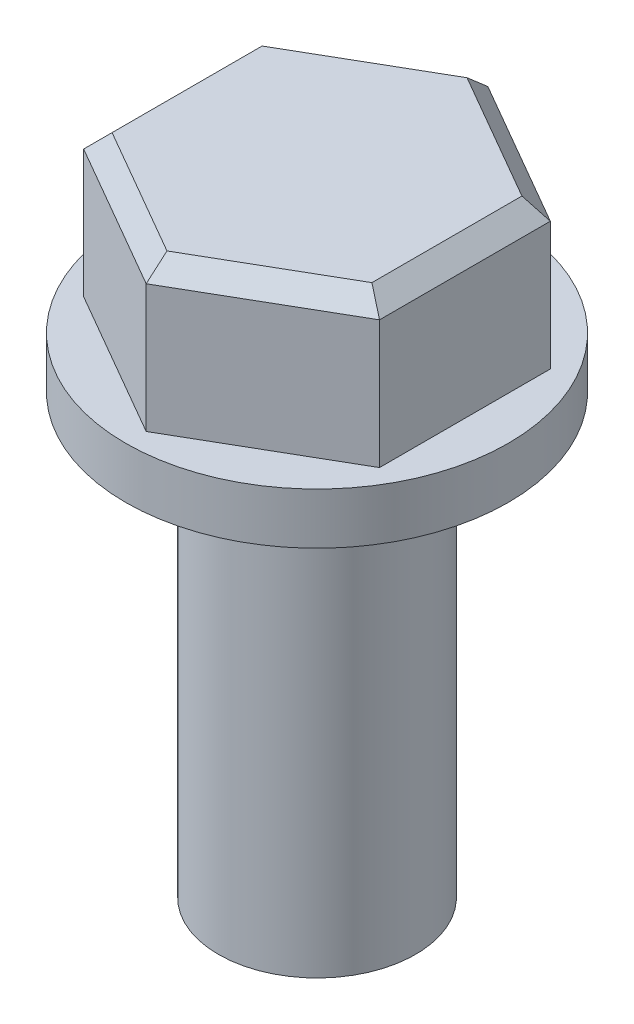
SolidWorks part; units mm, degrees
material "Plain Carbon Steel"
ref_plane "Front Plane" through (0, 0, 0) normal (0, 0, 1) x (1, 0, 0)
ref_plane "Top Plane" through (0, 0, 0) normal (0, 1, 0) x (1, 0, 0)
ref_plane "Right Plane" through (0, 0, 0) normal (1, 0, 0) x (0, 0, -1)
sketch "Shank Sketch Ø12.7" plane through (0, 0, 0) normal (0, 1, 0) x (1, 0, 0)
  circle A0 centre (0, 0) radius 6.35
  dimension "D1" = 12.7
extrude "Shank Ø12.7" add sketch "Shank Sketch Ø12.7" along normal blind 28.19
sketch "Flange Sketch Ø24.64" plane through (0, 28.19, 0) normal (0, 1, 0) x (1, 0, 0)
  circle A0 centre (0, 0) radius 12.32
  dimension "D1" = 24.64
extrude "Flange Ø24.64" add sketch "Flange Sketch Ø24.64" along normal blind 3.3
sketch "Hex Head Sketch" plane through (0, 31.49, 0) normal (0, 1, 0) x (1, 0, 0)
  line L1 (0, 11) -> (-9.5263, 5.5)
  line L2 (-9.5263, 5.5) -> (-9.5263, -5.5)
  line L3 (-9.5263, -5.5) -> (0, -11)
  line L4 (0, -11) -> (9.5263, -5.5)
  line L5 (9.5263, -5.5) -> (9.5263, 5.5)
  line L6 (9.5263, 5.5) -> (0, 11)
  circle A0 centre (0, 0) radius 11 construction
  dimension "D1" = 22
  dimension "D2" = 9.5263
extrude "Hex Head" add sketch "Hex Head Sketch" along normal blind 9.4
chamfer "Edge Chamfer 1.16x45 A" distance 1.16 angle 45 2 edges at (-9.5263, 40.89, 0) (-4.7631, 40.89, 8.25)
chamfer "Edge Chamfer 1.16x45 B" distance 1.16 angle 45 3 edges at (4.7631, 40.89, -8.25) (9.5263, 40.89, 0) (5.3431, 40.89, 7.9151)
chamfer "Edge Chamfer 1.16x45 C" distance 1.16 angle 45 1 edges at (-4.7631, 40.89, -8.25)
